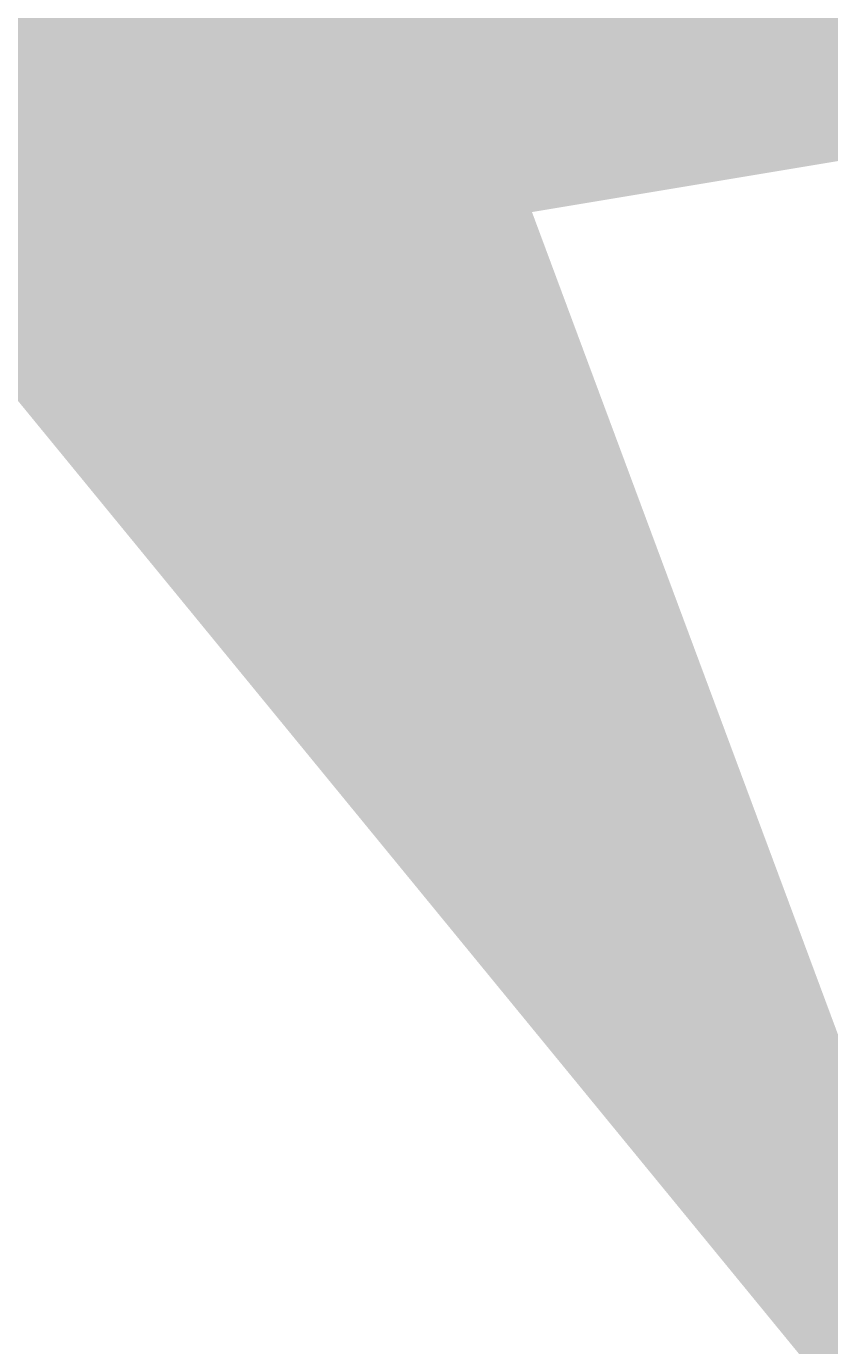
# Model space of a CAD drawing. Units: millimetres. Extents: x -22994 to 29398, y -19990 to 20176.
# Tile 21 of 135: x -44 to 5, y 99 to 180. Entities that reach past the tile are written whole.
import ezdxf

# ---------------------------------------------------------------- set-up
doc = ezdxf.new("R2010")
doc.units = ezdxf.units.MM
doc.header["$MEASUREMENT"] = 0
doc.layers.add('M-DIMS', color=2, linetype='Continuous', lineweight=18)
doc.styles.get("Standard").update_dxf_attribs({"font": 'arial.ttf'})
doc.dimstyles.get("Standard").update_dxf_attribs({"dimtxt": 0.18, "dimasz": 10000, "dimexe": 0.18, "dimexo": 0.0625, "dimgap": 0.09, "dimtad": 0, "dimtih": 1, "dimtoh": 1, "dimdec": 0, "dimzin": 0, "dimdsep": 46, "dimtxsty": 'Standard', "dimcen": 0.09, "dimadec": 0, "dimazin": 0, "dimtfac": 1, "dimtdec": 0, "dimtofl": 0, "dimtmove": 0, "dimatfit": 3, "dimfxl": 1, "dimtolj": 1, "dimtzin": 0, "dimlwd": 30, "dimarcsym": 0})

# ---------------------------------------------------------------- blocks, each defined once
blk = doc.blocks.new('*D2')
at = {"layer": 'Defpoints', "color": 0, "transparency": 16777216}
for p in [(6.677, 10.271), (290.852, 10.271), (290.852, -5.079)]:
    blk.add_point(p, dxfattribs=at)
at = {"layer": 'M-DIMS', "color": 0, "lineweight": -2, "transparency": 16777216}
for p, q in [((6.677, 10.209), (6.677, -5.259)), ((290.852, 10.209), (290.852, -5.259))]:
    blk.add_line(p, q, dxfattribs=at)
at = {"layer": 'M-DIMS', "color": 0, "lineweight": 30, "transparency": 16777216}
for p, q in [((-9993.323, -5.079), (-19993.323, -5.079)), ((10290.852, -5.079), (20290.852, -5.079))]:
    blk.add_line(p, q, dxfattribs=at)
at = {"layer": 'M-DIMS', "color": 0, "transparency": 16777216}
for points in [[(-9993.323, 1661.588), (-9993.323, -1671.745), (6.677, -5.079)], [(10290.852, 1661.588), (10290.852, -1671.745), (290.852, -5.079)]]:
    blk.add_solid(points, dxfattribs=at)
at = {"layer": 'M-DIMS', "color": 0, "transparency": 16777216, "insert": (148.765, -5.079), "char_height": 0.18, "attachment_point": 5}
blk.add_mtext('\\A1;284.2', dxfattribs=at)
blk = doc.blocks.new('*D3')
at = {"layer": 'Defpoints', "color": 0, "transparency": 16777216}
for p in [(110.265, 204.165), (110.265, 176.366), (95.833, 127.967)]:
    blk.add_point(p, dxfattribs=at)
at = {"layer": 'M-DIMS', "color": 0, "lineweight": 30, "transparency": 16777216}
for p, q in [((-9904.167, 204.165), (-19904.167, 204.165)), ((10110.265, 204.165), (20110.265, 204.165))]:
    blk.add_line(p, q, dxfattribs=at)
at = {"layer": 'M-DIMS', "color": 0, "lineweight": -2, "transparency": 16777216}
for p, q in [((95.833, 128.03), (95.833, 204.345)), ((110.265, 176.429), (110.265, 204.345))]:
    blk.add_line(p, q, dxfattribs=at)
at = {"layer": 'M-DIMS', "color": 0, "transparency": 16777216}
for points in [[(-9904.167, 1870.832), (-9904.167, -1462.501), (95.833, 204.165)], [(10110.265, 1870.832), (10110.265, -1462.501), (110.265, 204.165)]]:
    blk.add_solid(points, dxfattribs=at)
at = {"layer": 'M-DIMS', "color": 0, "transparency": 16777216, "insert": (103.049, 204.165), "char_height": 0.18, "attachment_point": 5}
blk.add_mtext('\\A1;14.432', dxfattribs=at)
blk = doc.blocks.new('*D4')
at = {"layer": 'Defpoints', "color": 0, "transparency": 16777216}
for p in [(116.265, 204.165), (110.265, 176.366), (116.265, 176.366)]:
    blk.add_point(p, dxfattribs=at)
at = {"layer": 'M-DIMS', "color": 0, "lineweight": 30, "transparency": 16777216}
for p, q in [((-9889.735, 204.165), (-19889.735, 204.165)), ((10116.265, 204.165), (20116.265, 204.165))]:
    blk.add_line(p, q, dxfattribs=at)
at = {"layer": 'M-DIMS', "color": 0, "lineweight": -2, "transparency": 16777216}
for p, q in [((110.265, 176.429), (110.265, 204.345)), ((116.265, 176.429), (116.265, 204.345))]:
    blk.add_line(p, q, dxfattribs=at)
at = {"layer": 'M-DIMS', "color": 0, "transparency": 16777216}
for points in [[(-9889.735, 1870.832), (-9889.735, -1462.501), (110.265, 204.165)], [(10116.265, 1870.832), (10116.265, -1462.501), (116.265, 204.165)]]:
    blk.add_solid(points, dxfattribs=at)
at = {"layer": 'M-DIMS', "color": 0, "transparency": 16777216, "insert": (113.265, 204.165), "char_height": 0.18, "attachment_point": 5}
blk.add_mtext('\\A1;6', dxfattribs=at)
blk = doc.blocks.new('*D5')
at = {"layer": 'Defpoints', "color": 0, "transparency": 16777216}
for p in [(181.265, 204.165), (116.265, 176.366), (181.265, 176.366)]:
    blk.add_point(p, dxfattribs=at)
at = {"layer": 'M-DIMS', "color": 0, "lineweight": 30, "transparency": 16777216}
for p, q in [((-9883.735, 204.165), (-19883.735, 204.165)), ((10181.265, 204.165), (20181.265, 204.165))]:
    blk.add_line(p, q, dxfattribs=at)
at = {"layer": 'M-DIMS', "color": 0, "lineweight": -2, "transparency": 16777216}
for p, q in [((116.265, 176.429), (116.265, 204.345)), ((181.265, 176.429), (181.265, 204.345))]:
    blk.add_line(p, q, dxfattribs=at)
at = {"layer": 'M-DIMS', "color": 0, "transparency": 16777216}
for points in [[(-9883.735, 1870.832), (-9883.735, -1462.501), (116.265, 204.165)], [(10181.265, 1870.832), (10181.265, -1462.501), (181.265, 204.165)]]:
    blk.add_solid(points, dxfattribs=at)
at = {"layer": 'M-DIMS', "color": 0, "transparency": 16777216, "insert": (148.765, 204.165), "char_height": 0.18, "attachment_point": 5}
blk.add_mtext('\\A1;65', dxfattribs=at)
blk = doc.blocks.new('*D6')
at = {"layer": 'Defpoints', "color": 0, "transparency": 16777216}
for p in [(187.265, 204.165), (181.265, 176.366), (187.265, 176.366)]:
    blk.add_point(p, dxfattribs=at)
at = {"layer": 'M-DIMS', "color": 0, "lineweight": 30, "transparency": 16777216}
for p, q in [((-9818.735, 204.165), (-19818.735, 204.165)), ((10187.265, 204.165), (20187.265, 204.165))]:
    blk.add_line(p, q, dxfattribs=at)
at = {"layer": 'M-DIMS', "color": 0, "lineweight": -2, "transparency": 16777216}
for p, q in [((181.265, 176.429), (181.265, 204.345)), ((187.265, 176.429), (187.265, 204.345))]:
    blk.add_line(p, q, dxfattribs=at)
at = {"layer": 'M-DIMS', "color": 0, "transparency": 16777216}
for points in [[(-9818.735, 1870.832), (-9818.735, -1462.501), (181.265, 204.165)], [(10187.265, 1870.832), (10187.265, -1462.501), (187.265, 204.165)]]:
    blk.add_solid(points, dxfattribs=at)
at = {"layer": 'M-DIMS', "color": 0, "transparency": 16777216, "insert": (184.265, 204.165), "char_height": 0.18, "attachment_point": 5}
blk.add_mtext('\\A1;6', dxfattribs=at)
blk = doc.blocks.new('*D7')
at = {"layer": 'Defpoints', "color": 0, "transparency": 16777216}
for p in [(201.697, 204.165), (187.265, 176.366), (201.697, 127.967)]:
    blk.add_point(p, dxfattribs=at)
at = {"layer": 'M-DIMS', "color": 0, "lineweight": 30, "transparency": 16777216}
for p, q in [((-9812.735, 204.165), (-19812.735, 204.165)), ((10201.697, 204.165), (20201.697, 204.165))]:
    blk.add_line(p, q, dxfattribs=at)
at = {"layer": 'M-DIMS', "color": 0, "lineweight": -2, "transparency": 16777216}
for p, q in [((187.265, 176.429), (187.265, 204.345)), ((201.697, 128.03), (201.697, 204.345))]:
    blk.add_line(p, q, dxfattribs=at)
at = {"layer": 'M-DIMS', "color": 0, "transparency": 16777216}
for points in [[(-9812.735, 1870.832), (-9812.735, -1462.501), (187.265, 204.165)], [(10201.697, 1870.832), (10201.697, -1462.501), (201.697, 204.165)]]:
    blk.add_solid(points, dxfattribs=at)
at = {"layer": 'M-DIMS', "color": 0, "transparency": 16777216, "insert": (194.481, 204.165), "char_height": 0.18, "attachment_point": 5}
blk.add_mtext('\\A1;14.432', dxfattribs=at)
blk = doc.blocks.new('*D8')
at = {"layer": 'Defpoints', "color": 0, "transparency": 16777216}
for p in [(227.648, 204.165), (227.648, 146.73), (201.697, 127.967)]:
    blk.add_point(p, dxfattribs=at)
at = {"layer": 'M-DIMS', "color": 0, "lineweight": 30, "transparency": 16777216}
for p, q in [((-9798.303, 204.165), (-19798.303, 204.165)), ((10227.648, 204.165), (20227.648, 204.165))]:
    blk.add_line(p, q, dxfattribs=at)
at = {"layer": 'M-DIMS', "color": 0, "lineweight": -2, "transparency": 16777216}
for p, q in [((201.697, 128.03), (201.697, 204.345)), ((227.648, 146.792), (227.648, 204.345))]:
    blk.add_line(p, q, dxfattribs=at)
at = {"layer": 'M-DIMS', "color": 0, "transparency": 16777216}
for points in [[(-9798.303, 1870.832), (-9798.303, -1462.501), (201.697, 204.165)], [(10227.648, 1870.832), (10227.648, -1462.501), (227.648, 204.165)]]:
    blk.add_solid(points, dxfattribs=at)
at = {"layer": 'M-DIMS', "color": 0, "transparency": 16777216, "insert": (214.673, 204.165), "char_height": 0.18, "attachment_point": 5}
blk.add_mtext('\\A1;25.95', dxfattribs=at)
blk = doc.blocks.new('*D9')
at = {"layer": 'Defpoints', "color": 0, "transparency": 16777216}
for p in [(187.265, 176.366), (306.202, 176.366), (290.852, 10.271)]:
    blk.add_point(p, dxfattribs=at)
at = {"layer": 'M-DIMS', "color": 0, "lineweight": 30, "transparency": 16777216}
for p, q in [((306.202, 10176.366), (306.202, 20176.366)), ((306.202, -9989.729), (306.202, -19989.729))]:
    blk.add_line(p, q, dxfattribs=at)
at = {"layer": 'M-DIMS', "color": 0, "lineweight": -2, "transparency": 16777216}
for p, q in [((187.327, 176.366), (306.382, 176.366)), ((290.915, 10.271), (306.382, 10.271))]:
    blk.add_line(p, q, dxfattribs=at)
at = {"layer": 'M-DIMS', "color": 0, "transparency": 16777216}
for points in [[(-1360.465, 10176.366), (1972.869, 10176.366), (306.202, 176.366)], [(-1360.465, -9989.729), (1972.869, -9989.729), (306.202, 10.271)]]:
    blk.add_solid(points, dxfattribs=at)
at = {"layer": 'M-DIMS', "color": 0, "transparency": 16777216, "insert": (306.202, 93.319), "char_height": 0.18, "attachment_point": 5}
blk.add_mtext('\\A1;166.1', dxfattribs=at)
blk = doc.blocks.new('*D10')
at = {"layer": 'Defpoints', "color": 0, "transparency": 16777216}
for p in [(125.65, 136.071), (133.346, 136.071), (133.346, -5.079)]:
    blk.add_point(p, dxfattribs=at)
at = {"layer": 'M-DIMS', "color": 0, "lineweight": -2, "transparency": 16777216}
for p, q in [((125.65, 136.009), (125.65, -5.259)), ((133.346, 136.009), (133.346, -5.259))]:
    blk.add_line(p, q, dxfattribs=at)
at = {"layer": 'M-DIMS', "color": 0, "lineweight": 30, "transparency": 16777216}
for p, q in [((-9874.35, -5.079), (-19874.35, -5.079)), ((10133.346, -5.079), (20133.346, -5.079))]:
    blk.add_line(p, q, dxfattribs=at)
at = {"layer": 'M-DIMS', "color": 0, "transparency": 16777216}
for points in [[(-9874.35, 1661.588), (-9874.35, -1671.745), (125.65, -5.079)], [(10133.346, 1661.588), (10133.346, -1671.745), (133.346, -5.079)]]:
    blk.add_solid(points, dxfattribs=at)
at = {"layer": 'M-DIMS', "color": 0, "transparency": 16777216, "insert": (129.498, -5.079), "char_height": 0.18, "attachment_point": 5}
blk.add_mtext('\\A1;7.696', dxfattribs=at)
blk = doc.blocks.new('*D11')
at = {"layer": 'Defpoints', "color": 0, "transparency": 16777216}
for p in [(133.346, 136.071), (135.65, 136.071), (135.65, -5.079)]:
    blk.add_point(p, dxfattribs=at)
at = {"layer": 'M-DIMS', "color": 0, "lineweight": -2, "transparency": 16777216}
for p, q in [((133.346, 136.009), (133.346, -5.259)), ((135.65, 136.009), (135.65, -5.259))]:
    blk.add_line(p, q, dxfattribs=at)
at = {"layer": 'M-DIMS', "color": 0, "lineweight": 30, "transparency": 16777216}
for p, q in [((-9866.654, -5.079), (-19866.654, -5.079)), ((10135.65, -5.079), (20135.65, -5.079))]:
    blk.add_line(p, q, dxfattribs=at)
at = {"layer": 'M-DIMS', "color": 0, "transparency": 16777216}
for points in [[(-9866.654, 1661.588), (-9866.654, -1671.745), (133.346, -5.079)], [(10135.65, 1661.588), (10135.65, -1671.745), (135.65, -5.079)]]:
    blk.add_solid(points, dxfattribs=at)
at = {"layer": 'M-DIMS', "color": 0, "transparency": 16777216, "insert": (134.498, -5.079), "char_height": 0.18, "attachment_point": 5}
blk.add_mtext('\\A1;2.304', dxfattribs=at)
blk = doc.blocks.new('*D12')
at = {"layer": 'Defpoints', "color": 0, "transparency": 16777216}
for p in [(135.65, 136.071), (145.65, 136.071), (145.65, -5.079)]:
    blk.add_point(p, dxfattribs=at)
at = {"layer": 'M-DIMS', "color": 0, "lineweight": -2, "transparency": 16777216}
for p, q in [((135.65, 136.009), (135.65, -5.259)), ((145.65, 136.009), (145.65, -5.259))]:
    blk.add_line(p, q, dxfattribs=at)
at = {"layer": 'M-DIMS', "color": 0, "lineweight": 30, "transparency": 16777216}
for p, q in [((-9864.35, -5.079), (-19864.35, -5.079)), ((10145.65, -5.079), (20145.65, -5.079))]:
    blk.add_line(p, q, dxfattribs=at)
at = {"layer": 'M-DIMS', "color": 0, "transparency": 16777216}
for points in [[(-9864.35, 1661.588), (-9864.35, -1671.745), (135.65, -5.079)], [(10145.65, 1661.588), (10145.65, -1671.745), (145.65, -5.079)]]:
    blk.add_solid(points, dxfattribs=at)
at = {"layer": 'M-DIMS', "color": 0, "transparency": 16777216, "insert": (140.65, -5.079), "char_height": 0.18, "attachment_point": 5}
blk.add_mtext('\\A1;10', dxfattribs=at)
blk = doc.blocks.new('*D13')
at = {"layer": 'Defpoints', "color": 0, "transparency": 16777216}
for p in [(145.65, 136.071), (155.65, 136.071), (155.65, -5.079)]:
    blk.add_point(p, dxfattribs=at)
at = {"layer": 'M-DIMS', "color": 0, "lineweight": -2, "transparency": 16777216}
for p, q in [((145.65, 136.009), (145.65, -5.259)), ((155.65, 136.009), (155.65, -5.259))]:
    blk.add_line(p, q, dxfattribs=at)
at = {"layer": 'M-DIMS', "color": 0, "lineweight": 30, "transparency": 16777216}
for p, q in [((-9854.35, -5.079), (-19854.35, -5.079)), ((10155.65, -5.079), (20155.65, -5.079))]:
    blk.add_line(p, q, dxfattribs=at)
at = {"layer": 'M-DIMS', "color": 0, "transparency": 16777216}
for points in [[(-9854.35, 1661.588), (-9854.35, -1671.745), (145.65, -5.079)], [(10155.65, 1661.588), (10155.65, -1671.745), (155.65, -5.079)]]:
    blk.add_solid(points, dxfattribs=at)
at = {"layer": 'M-DIMS', "color": 0, "transparency": 16777216, "insert": (150.65, -5.079), "char_height": 0.18, "attachment_point": 5}
blk.add_mtext('\\A1;10', dxfattribs=at)
blk = doc.blocks.new('*D14')
at = {"layer": 'Defpoints', "color": 0, "transparency": 16777216}
for p in [(155.65, 136.071), (165.65, 136.071), (165.65, -5.079)]:
    blk.add_point(p, dxfattribs=at)
at = {"layer": 'M-DIMS', "color": 0, "lineweight": -2, "transparency": 16777216}
for p, q in [((155.65, 136.009), (155.65, -5.259)), ((165.65, 136.009), (165.65, -5.259))]:
    blk.add_line(p, q, dxfattribs=at)
at = {"layer": 'M-DIMS', "color": 0, "lineweight": 30, "transparency": 16777216}
for p, q in [((-9844.35, -5.079), (-19844.35, -5.079)), ((10165.65, -5.079), (20165.65, -5.079))]:
    blk.add_line(p, q, dxfattribs=at)
at = {"layer": 'M-DIMS', "color": 0, "transparency": 16777216}
for points in [[(-9844.35, 1661.588), (-9844.35, -1671.745), (155.65, -5.079)], [(10165.65, 1661.588), (10165.65, -1671.745), (165.65, -5.079)]]:
    blk.add_solid(points, dxfattribs=at)
at = {"layer": 'M-DIMS', "color": 0, "transparency": 16777216, "insert": (160.65, -5.079), "char_height": 0.18, "attachment_point": 5}
blk.add_mtext('\\A1;10', dxfattribs=at)
blk = doc.blocks.new('*D15')
at = {"layer": 'Defpoints', "color": 0, "transparency": 16777216}
for p in [(173.346, 154.788), (173.346, 136.071), (306.202, 136.071)]:
    blk.add_point(p, dxfattribs=at)
at = {"layer": 'M-DIMS', "color": 0, "lineweight": 30, "transparency": 16777216}
for p, q in [((306.202, 10154.788), (306.202, 20154.788)), ((306.202, -9863.929), (306.202, -19863.929))]:
    blk.add_line(p, q, dxfattribs=at)
at = {"layer": 'M-DIMS', "color": 0, "lineweight": -2, "transparency": 16777216}
for p, q in [((173.408, 154.788), (306.382, 154.788)), ((173.408, 136.071), (306.382, 136.071))]:
    blk.add_line(p, q, dxfattribs=at)
at = {"layer": 'M-DIMS', "color": 0, "transparency": 16777216}
for points in [[(-1360.465, 10154.788), (1972.869, 10154.788), (306.202, 154.788)], [(-1360.465, -9863.929), (1972.869, -9863.929), (306.202, 136.071)]]:
    blk.add_solid(points, dxfattribs=at)
at = {"layer": 'M-DIMS', "color": 0, "transparency": 16777216, "insert": (306.202, 145.43), "char_height": 0.18, "attachment_point": 5}
blk.add_mtext('\\A1;18.717', dxfattribs=at)
blk = doc.blocks.new('*D16')
at = {"layer": 'Defpoints', "color": 0, "transparency": 16777216}
for p in [(120.17, 204.165), (110.466, 48.035), (120.17, 48.035)]:
    blk.add_point(p, dxfattribs=at)
at = {"layer": 'M-DIMS', "color": 0, "lineweight": 30, "transparency": 16777216}
for p, q in [((-9889.534, 204.165), (-19889.534, 204.165)), ((10120.17, 204.165), (20120.17, 204.165))]:
    blk.add_line(p, q, dxfattribs=at)
at = {"layer": 'M-DIMS', "color": 0, "lineweight": -2, "transparency": 16777216}
for p, q in [((110.466, 48.097), (110.466, 204.345)), ((120.17, 48.097), (120.17, 204.345))]:
    blk.add_line(p, q, dxfattribs=at)
at = {"layer": 'M-DIMS', "color": 0, "transparency": 16777216}
for points in [[(-9889.534, 1870.832), (-9889.534, -1462.501), (110.466, 204.165)], [(10120.17, 1870.832), (10120.17, -1462.501), (120.17, 204.165)]]:
    blk.add_solid(points, dxfattribs=at)
at = {"layer": 'M-DIMS', "color": 0, "transparency": 16777216, "insert": (115.318, 204.165), "char_height": 0.18, "attachment_point": 5}
blk.add_mtext('\\A1;9.704', dxfattribs=at)
blk = doc.blocks.new('*D17')
at = {"layer": 'Defpoints', "color": 0, "transparency": 16777216}
for p in [(126.17, 204.165), (120.17, 48.035), (126.17, 48.035)]:
    blk.add_point(p, dxfattribs=at)
at = {"layer": 'M-DIMS', "color": 0, "lineweight": 30, "transparency": 16777216}
for p, q in [((-9879.83, 204.165), (-19879.83, 204.165)), ((10126.17, 204.165), (20126.17, 204.165))]:
    blk.add_line(p, q, dxfattribs=at)
at = {"layer": 'M-DIMS', "color": 0, "lineweight": -2, "transparency": 16777216}
for p, q in [((120.17, 48.097), (120.17, 204.345)), ((126.17, 48.097), (126.17, 204.345))]:
    blk.add_line(p, q, dxfattribs=at)
at = {"layer": 'M-DIMS', "color": 0, "transparency": 16777216}
for points in [[(-9879.83, 1870.832), (-9879.83, -1462.501), (120.17, 204.165)], [(10126.17, 1870.832), (10126.17, -1462.501), (126.17, 204.165)]]:
    blk.add_solid(points, dxfattribs=at)
at = {"layer": 'M-DIMS', "color": 0, "transparency": 16777216, "insert": (123.17, 204.165), "char_height": 0.18, "attachment_point": 5}
blk.add_mtext('\\A1;6', dxfattribs=at)
blk = doc.blocks.new('*D18')
at = {"layer": 'Defpoints', "color": 0, "transparency": 16777216}
for p in [(132.17, 204.165), (126.17, 48.035), (132.17, 48.035)]:
    blk.add_point(p, dxfattribs=at)
at = {"layer": 'M-DIMS', "color": 0, "lineweight": 30, "transparency": 16777216}
for p, q in [((-9873.83, 204.165), (-19873.83, 204.165)), ((10132.17, 204.165), (20132.17, 204.165))]:
    blk.add_line(p, q, dxfattribs=at)
at = {"layer": 'M-DIMS', "color": 0, "lineweight": -2, "transparency": 16777216}
for p, q in [((126.17, 48.097), (126.17, 204.345)), ((132.17, 48.097), (132.17, 204.345))]:
    blk.add_line(p, q, dxfattribs=at)
at = {"layer": 'M-DIMS', "color": 0, "transparency": 16777216}
for points in [[(-9873.83, 1870.832), (-9873.83, -1462.501), (126.17, 204.165)], [(10132.17, 1870.832), (10132.17, -1462.501), (132.17, 204.165)]]:
    blk.add_solid(points, dxfattribs=at)
at = {"layer": 'M-DIMS', "color": 0, "transparency": 16777216, "insert": (129.17, 204.165), "char_height": 0.18, "attachment_point": 5}
blk.add_mtext('\\A1;6', dxfattribs=at)
blk = doc.blocks.new('*D19')
at = {"layer": 'Defpoints', "color": 0, "transparency": 16777216}
for p in [(138.17, 204.165), (132.17, 48.035), (138.17, 48.035)]:
    blk.add_point(p, dxfattribs=at)
at = {"layer": 'M-DIMS', "color": 0, "lineweight": 30, "transparency": 16777216}
for p, q in [((-9867.83, 204.165), (-19867.83, 204.165)), ((10138.17, 204.165), (20138.17, 204.165))]:
    blk.add_line(p, q, dxfattribs=at)
at = {"layer": 'M-DIMS', "color": 0, "lineweight": -2, "transparency": 16777216}
for p, q in [((132.17, 48.097), (132.17, 204.345)), ((138.17, 48.097), (138.17, 204.345))]:
    blk.add_line(p, q, dxfattribs=at)
at = {"layer": 'M-DIMS', "color": 0, "transparency": 16777216}
for points in [[(-9867.83, 1870.832), (-9867.83, -1462.501), (132.17, 204.165)], [(10138.17, 1870.832), (10138.17, -1462.501), (138.17, 204.165)]]:
    blk.add_solid(points, dxfattribs=at)
at = {"layer": 'M-DIMS', "color": 0, "transparency": 16777216, "insert": (135.17, 204.165), "char_height": 0.18, "attachment_point": 5}
blk.add_mtext('\\A1;6', dxfattribs=at)
blk = doc.blocks.new('*D20')
at = {"layer": 'Defpoints', "color": 0, "transparency": 16777216}
for p in [(144.17, 204.165), (138.17, 48.035), (144.17, 48.035)]:
    blk.add_point(p, dxfattribs=at)
at = {"layer": 'M-DIMS', "color": 0, "lineweight": 30, "transparency": 16777216}
for p, q in [((-9861.83, 204.165), (-19861.83, 204.165)), ((10144.17, 204.165), (20144.17, 204.165))]:
    blk.add_line(p, q, dxfattribs=at)
at = {"layer": 'M-DIMS', "color": 0, "lineweight": -2, "transparency": 16777216}
for p, q in [((138.17, 48.097), (138.17, 204.345)), ((144.17, 48.097), (144.17, 204.345))]:
    blk.add_line(p, q, dxfattribs=at)
at = {"layer": 'M-DIMS', "color": 0, "transparency": 16777216}
for points in [[(-9861.83, 1870.832), (-9861.83, -1462.501), (138.17, 204.165)], [(10144.17, 1870.832), (10144.17, -1462.501), (144.17, 204.165)]]:
    blk.add_solid(points, dxfattribs=at)
at = {"layer": 'M-DIMS', "color": 0, "transparency": 16777216, "insert": (141.17, 204.165), "char_height": 0.18, "attachment_point": 5}
blk.add_mtext('\\A1;6', dxfattribs=at)
blk = doc.blocks.new('*D21')
at = {"layer": 'Defpoints', "color": 0, "transparency": 16777216}
for p in [(149.116, 204.165), (144.17, 48.035), (149.116, 48.035)]:
    blk.add_point(p, dxfattribs=at)
at = {"layer": 'M-DIMS', "color": 0, "lineweight": 30, "transparency": 16777216}
for p, q in [((-9855.83, 204.165), (-19855.83, 204.165)), ((10149.116, 204.165), (20149.116, 204.165))]:
    blk.add_line(p, q, dxfattribs=at)
at = {"layer": 'M-DIMS', "color": 0, "lineweight": -2, "transparency": 16777216}
for p, q in [((144.17, 48.097), (144.17, 204.345)), ((149.116, 48.097), (149.116, 204.345))]:
    blk.add_line(p, q, dxfattribs=at)
at = {"layer": 'M-DIMS', "color": 0, "transparency": 16777216}
for points in [[(-9855.83, 1870.832), (-9855.83, -1462.501), (144.17, 204.165)], [(10149.116, 1870.832), (10149.116, -1462.501), (149.116, 204.165)]]:
    blk.add_solid(points, dxfattribs=at)
at = {"layer": 'M-DIMS', "color": 0, "transparency": 16777216, "insert": (146.643, 204.165), "char_height": 0.18, "attachment_point": 5}
blk.add_mtext('\\A1;4.945', dxfattribs=at)
blk = doc.blocks.new('*D22')
at = {"layer": 'Defpoints', "color": 0, "transparency": 16777216}
for p in [(149.116, 30.99), (155.116, 30.99), (155.116, -5.079)]:
    blk.add_point(p, dxfattribs=at)
at = {"layer": 'M-DIMS', "color": 0, "lineweight": -2, "transparency": 16777216}
for p, q in [((149.116, 30.927), (149.116, -5.259)), ((155.116, 30.927), (155.116, -5.259))]:
    blk.add_line(p, q, dxfattribs=at)
at = {"layer": 'M-DIMS', "color": 0, "lineweight": 30, "transparency": 16777216}
for p, q in [((-9850.884, -5.079), (-19850.884, -5.079)), ((10155.116, -5.079), (20155.116, -5.079))]:
    blk.add_line(p, q, dxfattribs=at)
at = {"layer": 'M-DIMS', "color": 0, "transparency": 16777216}
for points in [[(-9850.884, 1661.588), (-9850.884, -1671.745), (149.116, -5.079)], [(10155.116, 1661.588), (10155.116, -1671.745), (155.116, -5.079)]]:
    blk.add_solid(points, dxfattribs=at)
at = {"layer": 'M-DIMS', "color": 0, "transparency": 16777216, "insert": (152.116, -5.079), "char_height": 0.18, "attachment_point": 5}
blk.add_mtext('\\A1;6', dxfattribs=at)
blk = doc.blocks.new('*D23')
at = {"layer": 'Defpoints', "color": 0, "transparency": 16777216}
for p in [(155.116, 30.99), (161.116, 30.99), (161.116, -5.079)]:
    blk.add_point(p, dxfattribs=at)
at = {"layer": 'M-DIMS', "color": 0, "lineweight": -2, "transparency": 16777216}
for p, q in [((155.116, 30.927), (155.116, -5.259)), ((161.116, 30.927), (161.116, -5.259))]:
    blk.add_line(p, q, dxfattribs=at)
at = {"layer": 'M-DIMS', "color": 0, "lineweight": 30, "transparency": 16777216}
for p, q in [((-9844.884, -5.079), (-19844.884, -5.079)), ((10161.116, -5.079), (20161.116, -5.079))]:
    blk.add_line(p, q, dxfattribs=at)
at = {"layer": 'M-DIMS', "color": 0, "transparency": 16777216}
for points in [[(-9844.884, 1661.588), (-9844.884, -1671.745), (155.116, -5.079)], [(10161.116, 1661.588), (10161.116, -1671.745), (161.116, -5.079)]]:
    blk.add_solid(points, dxfattribs=at)
at = {"layer": 'M-DIMS', "color": 0, "transparency": 16777216, "insert": (158.116, -5.079), "char_height": 0.18, "attachment_point": 5}
blk.add_mtext('\\A1;6', dxfattribs=at)
blk = doc.blocks.new('*D24')
at = {"layer": 'Defpoints', "color": 0, "transparency": 16777216}
for p in [(161.116, 30.99), (166.439, 30.99), (166.439, -5.079)]:
    blk.add_point(p, dxfattribs=at)
at = {"layer": 'M-DIMS', "color": 0, "lineweight": -2, "transparency": 16777216}
for p, q in [((161.116, 30.927), (161.116, -5.259)), ((166.439, 30.927), (166.439, -5.259))]:
    blk.add_line(p, q, dxfattribs=at)
at = {"layer": 'M-DIMS', "color": 0, "lineweight": 30, "transparency": 16777216}
for p, q in [((-9838.884, -5.079), (-19838.884, -5.079)), ((10166.439, -5.079), (20166.439, -5.079))]:
    blk.add_line(p, q, dxfattribs=at)
at = {"layer": 'M-DIMS', "color": 0, "transparency": 16777216}
for points in [[(-9838.884, 1661.588), (-9838.884, -1671.745), (161.116, -5.079)], [(10166.439, 1661.588), (10166.439, -1671.745), (166.439, -5.079)]]:
    blk.add_solid(points, dxfattribs=at)
at = {"layer": 'M-DIMS', "color": 0, "transparency": 16777216, "insert": (163.777, -5.079), "char_height": 0.18, "attachment_point": 5}
blk.add_mtext('\\A1;5.323', dxfattribs=at)
blk = doc.blocks.new('*D25')
at = {"layer": 'Defpoints', "color": 0, "transparency": 16777216}
for p in [(166.439, 30.99), (172.439, 30.99), (172.439, -5.079)]:
    blk.add_point(p, dxfattribs=at)
at = {"layer": 'M-DIMS', "color": 0, "lineweight": -2, "transparency": 16777216}
for p, q in [((166.439, 30.927), (166.439, -5.259)), ((172.439, 30.927), (172.439, -5.259))]:
    blk.add_line(p, q, dxfattribs=at)
at = {"layer": 'M-DIMS', "color": 0, "lineweight": 30, "transparency": 16777216}
for p, q in [((-9833.561, -5.079), (-19833.561, -5.079)), ((10172.439, -5.079), (20172.439, -5.079))]:
    blk.add_line(p, q, dxfattribs=at)
at = {"layer": 'M-DIMS', "color": 0, "transparency": 16777216}
for points in [[(-9833.561, 1661.588), (-9833.561, -1671.745), (166.439, -5.079)], [(10172.439, 1661.588), (10172.439, -1671.745), (172.439, -5.079)]]:
    blk.add_solid(points, dxfattribs=at)
at = {"layer": 'M-DIMS', "color": 0, "transparency": 16777216, "insert": (169.439, -5.079), "char_height": 0.18, "attachment_point": 5}
blk.add_mtext('\\A1;6', dxfattribs=at)
blk = doc.blocks.new('*D26')
at = {"layer": 'Defpoints', "color": 0, "transparency": 16777216}
for p in [(172.439, 30.99), (178.439, 30.99), (178.439, -5.079)]:
    blk.add_point(p, dxfattribs=at)
at = {"layer": 'M-DIMS', "color": 0, "lineweight": -2, "transparency": 16777216}
for p, q in [((172.439, 30.927), (172.439, -5.259)), ((178.439, 30.927), (178.439, -5.259))]:
    blk.add_line(p, q, dxfattribs=at)
at = {"layer": 'M-DIMS', "color": 0, "lineweight": 30, "transparency": 16777216}
for p, q in [((-9827.561, -5.079), (-19827.561, -5.079)), ((10178.439, -5.079), (20178.439, -5.079))]:
    blk.add_line(p, q, dxfattribs=at)
at = {"layer": 'M-DIMS', "color": 0, "transparency": 16777216}
for points in [[(-9827.561, 1661.588), (-9827.561, -1671.745), (172.439, -5.079)], [(10178.439, 1661.588), (10178.439, -1671.745), (178.439, -5.079)]]:
    blk.add_solid(points, dxfattribs=at)
at = {"layer": 'M-DIMS', "color": 0, "transparency": 16777216, "insert": (175.439, -5.079), "char_height": 0.18, "attachment_point": 5}
blk.add_mtext('\\A1;6', dxfattribs=at)
blk = doc.blocks.new('*D27')
at = {"layer": 'Defpoints', "color": 0, "transparency": 16777216}
for p in [(178.439, 30.99), (188.117, 30.99), (188.117, -5.079)]:
    blk.add_point(p, dxfattribs=at)
at = {"layer": 'M-DIMS', "color": 0, "lineweight": -2, "transparency": 16777216}
for p, q in [((178.439, 30.927), (178.439, -5.259)), ((188.117, 30.927), (188.117, -5.259))]:
    blk.add_line(p, q, dxfattribs=at)
at = {"layer": 'M-DIMS', "color": 0, "lineweight": 30, "transparency": 16777216}
for p, q in [((-9821.561, -5.079), (-19821.561, -5.079)), ((10188.117, -5.079), (20188.117, -5.079))]:
    blk.add_line(p, q, dxfattribs=at)
at = {"layer": 'M-DIMS', "color": 0, "transparency": 16777216}
for points in [[(-9821.561, 1661.588), (-9821.561, -1671.745), (178.439, -5.079)], [(10188.117, 1661.588), (10188.117, -1671.745), (188.117, -5.079)]]:
    blk.add_solid(points, dxfattribs=at)
at = {"layer": 'M-DIMS', "color": 0, "transparency": 16777216, "insert": (183.278, -5.079), "char_height": 0.18, "attachment_point": 5}
blk.add_mtext('\\A1;9.679', dxfattribs=at)
blk = doc.blocks.new('*D28')
at = {"layer": 'Defpoints', "color": 0, "transparency": 16777216}
for p in [(188.117, 48.035), (306.202, 48.035), (188.117, 30.99)]:
    blk.add_point(p, dxfattribs=at)
at = {"layer": 'M-DIMS', "color": 0, "lineweight": 30, "transparency": 16777216}
for p, q in [((306.202, 10048.035), (306.202, 20048.035)), ((306.202, -9969.01), (306.202, -19969.01))]:
    blk.add_line(p, q, dxfattribs=at)
at = {"layer": 'M-DIMS', "color": 0, "lineweight": -2, "transparency": 16777216}
for p, q in [((188.18, 48.035), (306.382, 48.035)), ((188.18, 30.99), (306.382, 30.99))]:
    blk.add_line(p, q, dxfattribs=at)
at = {"layer": 'M-DIMS', "color": 0, "transparency": 16777216}
for points in [[(-1360.465, 10048.035), (1972.869, 10048.035), (306.202, 48.035)], [(-1360.465, -9969.01), (1972.869, -9969.01), (306.202, 30.99)]]:
    blk.add_solid(points, dxfattribs=at)
at = {"layer": 'M-DIMS', "color": 0, "transparency": 16777216, "insert": (306.202, 39.512), "char_height": 0.18, "attachment_point": 5}
blk.add_mtext('\\A1;17.045', dxfattribs=at)
blk = doc.blocks.new('*D32')
at = {"layer": 'Defpoints', "color": 0, "transparency": 16777216}
for p in [(57.164, 118.614), (52.413, 113.093)]:
    blk.add_point(p, dxfattribs=at)
at = {"layer": 'M-DIMS', "color": 0, "lineweight": -2, "transparency": 16777216}
for p, q in [((57.074, 118.614), (57.254, 118.614)), ((57.164, 118.524), (57.164, 118.704))]:
    blk.add_line(p, q, dxfattribs=at)
at = {"layer": 'M-DIMS', "color": 0, "lineweight": 30, "transparency": 16777216}
for p, q in [((-12992.534, -15047.031), (-6470.06, -7466.969)), ((-22992.534, -15047.031), (-12992.534, -15047.031))]:
    blk.add_line(p, q, dxfattribs=at)
at = {"layer": 'M-DIMS', "color": 0, "transparency": 16777216}
blk.add_solid([(-7733.404, -6379.89), (-5206.717, -8554.048), (52.413, 113.093)], dxfattribs=at)
at = {"layer": 'M-DIMS', "color": 0, "transparency": 16777216, "insert": (-22993.208, -15047.031), "char_height": 0.18, "attachment_point": 5}
blk.add_mtext('\\A1;2X R7.284', dxfattribs=at)
blk = doc.blocks.new('*D35')
at = {"layer": 'Defpoints', "color": 0, "transparency": 16777216}
for p in [(21.093, 77.393), (21.84, 76.092)]:
    blk.add_point(p, dxfattribs=at)
at = {"layer": 'M-DIMS', "color": 0, "lineweight": 30, "transparency": 16777216}
for p, q in [((-19938.013, 17421.447), (-9938.013, 17421.447)), ((-9938.013, 17421.447), (-4958.46, 8749.42))]:
    blk.add_line(p, q, dxfattribs=at)
at = {"layer": 'M-DIMS', "color": 0, "lineweight": -2, "transparency": 16777216}
for p, q in [((21.75, 76.092), (21.93, 76.092)), ((21.84, 76.002), (21.84, 76.182))]:
    blk.add_line(p, q, dxfattribs=at)
at = {"layer": 'M-DIMS', "color": 0, "transparency": 16777216}
blk.add_solid([(-3513.122, 9579.345), (-6403.798, 7919.494), (21.093, 77.393)], dxfattribs=at)
at = {"layer": 'M-DIMS', "color": 0, "transparency": 16777216, "insert": (-19938.354, 17421.447), "char_height": 0.18, "attachment_point": 5}
blk.add_mtext('\\A1;R1.5', dxfattribs=at)
blk = doc.blocks.new('*D36')
at = {"layer": 'Defpoints', "color": 0, "transparency": 16777216}
for p in [(46.39, 31.303), (46.387, 26.593)]:
    blk.add_point(p, dxfattribs=at)
at = {"layer": 'M-DIMS', "color": 0, "lineweight": 30, "transparency": 16777216}
for p, q in [((57.15, 20031.301), (51.77, 10031.302)), ((10057.15, 20031.301), (57.15, 20031.301))]:
    blk.add_line(p, q, dxfattribs=at)
at = {"layer": 'M-DIMS', "color": 0, "lineweight": -2, "transparency": 16777216}
for p, q in [((46.299, 28.948), (46.479, 28.948)), ((46.389, 28.858), (46.389, 29.038))]:
    blk.add_line(p, q, dxfattribs=at)
at = {"layer": 'M-DIMS', "color": 0, "transparency": 16777216}
blk.add_solid([(-1614.896, 10032.199), (1718.436, 10030.405), (46.39, 31.303)], dxfattribs=at)
at = {"layer": 'M-DIMS', "color": 0, "transparency": 16777216, "insert": (10057.554, 20031.301), "char_height": 0.18, "attachment_point": 5}
blk.add_mtext('\\A1;∅4.71', dxfattribs=at)

msp = doc.modelspace()

# ---------------------------------------------------------------- dimensions: what is measured, and where the dimension line sits
at = {"layer": 'M-DIMS'}
for base, p1, p2, override, picture, middle in [((306.202, 176.3662), (290.852, 10.2713), (187.2647, 176.3662), {"dimdec": 1, "dimlfac": 1, "dimrnd": 0, "dimzin": 0, "dimdsep": 46, "dimlunit": 2}, '*D9', (306.202, 93.3187)), ((306.202, 136.0713), (173.3459, 154.788), (173.3459, 136.0713), {"dimdec": 3, "dimlfac": 1, "dimrnd": 0, "dimzin": 0, "dimdsep": 46, "dimlunit": 2}, '*D15', (306.202, 145.4297)), ((306.202, 48.0349), (188.1175, 30.9895), (188.1175, 48.0349), {"dimdec": 3, "dimlfac": 1, "dimrnd": 0, "dimzin": 0, "dimdsep": 46, "dimlunit": 2}, '*D28', (306.202, 39.5122))]:
    dim = msp.add_linear_dim(base=base, p1=p1, p2=p2, angle=90, dimstyle='Standard', override=override, dxfattribs=at)
    dim.commit()
    dim.dimension.update_dxf_attribs({"geometry": picture, "text_midpoint": middle})
dim = msp.add_diameter_dim_2p(p1=(46.3875, 26.5934), p2=(46.39, 31.3035), dimstyle='Standard', override={"dimdec": 2, "dimlfac": 1, "dimrnd": 0, "dimzin": 0, "dimdsep": 46, "dimlunit": 2}, dxfattribs=at)
dim.commit()
dim.dimension.update_dxf_attribs({"geometry": '*D36', "text_midpoint": (10057.5542, 20031.3006), "dimtype": 163})
dim = msp.add_radius_dim(center=(21.8402, 76.0922), mpoint=(21.0933, 77.393), dimstyle='Standard', override={"dimdec": 1, "dimlfac": 1, "dimrnd": 0, "dimzin": 0, "dimdsep": 46, "dimlunit": 2}, dxfattribs=at)
dim.commit()
dim.dimension.update_dxf_attribs({"geometry": '*D35', "text_midpoint": (-19938.3541, 17421.4466)})
for base, p1, p2, override, picture, middle in [((110.2647, 204.1654), (95.8327, 127.967), (110.2647, 176.3662), {"dimdec": 3, "dimlfac": 1, "dimrnd": 0, "dimzin": 0, "dimdsep": 46, "dimlunit": 2}, '*D3', (103.0487, 204.1654)), ((116.2647, 204.1654), (110.2647, 176.3662), (116.2647, 176.3662), {"dimdec": 0, "dimlfac": 1, "dimrnd": 0, "dimzin": 0, "dimdsep": 46, "dimlunit": 2}, '*D4', (113.2647, 204.1654)), ((120.1702, 204.1654), (110.4658, 48.0349), (120.1702, 48.0349), {"dimdec": 3, "dimlfac": 1, "dimrnd": 0, "dimzin": 0, "dimdsep": 46, "dimlunit": 2}, '*D16', (115.318, 204.1654)), ((181.2647, 204.1654), (116.2647, 176.3662), (181.2647, 176.3662), {"dimdec": 0, "dimlfac": 1, "dimrnd": 0, "dimzin": 0, "dimdsep": 46, "dimlunit": 2}, '*D5', (148.7647, 204.1654)), ((126.1702, 204.1654), (120.1702, 48.0349), (126.1702, 48.0349), {"dimdec": 0, "dimlfac": 1, "dimrnd": 0, "dimzin": 0, "dimdsep": 46, "dimlunit": 2}, '*D17', (123.1702, 204.1654)), ((132.1702, 204.1654), (126.1702, 48.0349), (132.1702, 48.0349), {"dimdec": 0, "dimlfac": 1, "dimrnd": 0, "dimzin": 0, "dimdsep": 46, "dimlunit": 2}, '*D18', (129.1702, 204.1654)), ((138.1702, 204.1654), (132.1702, 48.0349), (138.1702, 48.0349), {"dimdec": 0, "dimlfac": 1, "dimrnd": 0, "dimzin": 0, "dimdsep": 46, "dimlunit": 2}, '*D19', (135.1702, 204.1654)), ((144.1702, 204.1654), (138.1702, 48.0349), (144.1702, 48.0349), {"dimdec": 0, "dimlfac": 1, "dimrnd": 0, "dimzin": 0, "dimdsep": 46, "dimlunit": 2}, '*D20', (141.1702, 204.1654)), ((149.11567, 204.16539), (144.17023, 48.03494), (149.11567, 48.03494), {"dimdec": 3, "dimlfac": 1, "dimrnd": 0, "dimzin": 0, "dimdsep": 46, "dimlunit": 2}, '*D21', (146.64295, 204.16539)), ((187.2647, 204.1654), (181.2647, 176.3662), (187.2647, 176.3662), {"dimdec": 0, "dimlfac": 1, "dimrnd": 0, "dimzin": 0, "dimdsep": 46, "dimlunit": 2}, '*D6', (184.2647, 204.1654)), ((201.6967, 204.1654), (187.2647, 176.3662), (201.6967, 127.967), {"dimdec": 3, "dimlfac": 1, "dimrnd": 0, "dimzin": 0, "dimdsep": 46, "dimlunit": 2}, '*D7', (194.4807, 204.1654)), ((227.6485, 204.1654), (201.6967, 127.967), (227.6485, 146.7296), {"dimdec": 2, "dimlfac": 1, "dimrnd": 0, "dimzin": 0, "dimdsep": 46, "dimlunit": 2}, '*D8', (214.6726, 204.1654)), ((290.852, -5.0787), (6.6773, 10.2713), (290.852, 10.2713), {"dimdec": 1, "dimlfac": 1, "dimrnd": 0, "dimzin": 0, "dimdsep": 46, "dimlunit": 2}, '*D2', (148.7647, -5.0787)), ((133.3459, -5.0787), (125.6498, 136.0713), (133.3459, 136.0713), {"dimdec": 3, "dimlfac": 1, "dimrnd": 0, "dimzin": 0, "dimdsep": 46, "dimlunit": 2}, '*D10', (129.4978, -5.0787)), ((135.6498, -5.0787), (133.3459, 136.0713), (135.6498, 136.0713), {"dimdec": 3, "dimlfac": 1, "dimrnd": 0, "dimzin": 0, "dimdsep": 46, "dimlunit": 2}, '*D11', (134.4978, -5.0787)), ((145.6498, -5.0787), (135.6498, 136.0713), (145.6498, 136.0713), {"dimdec": 0, "dimlfac": 1, "dimrnd": 0, "dimzin": 0, "dimdsep": 46, "dimlunit": 2}, '*D12', (140.6498, -5.0787)), ((155.6498, -5.0787), (145.6498, 136.0713), (155.6498, 136.0713), {"dimdec": 0, "dimlfac": 1, "dimrnd": 0, "dimzin": 0, "dimdsep": 46, "dimlunit": 2}, '*D13', (150.6498, -5.0787)), ((155.1157, -5.0787), (149.1157, 30.9895), (155.1157, 30.9895), {"dimdec": 0, "dimlfac": 1, "dimrnd": 0, "dimzin": 0, "dimdsep": 46, "dimlunit": 2}, '*D22', (152.1157, -5.0787)), ((161.1157, -5.0787), (155.1157, 30.9895), (161.1157, 30.9895), {"dimdec": 0, "dimlfac": 1, "dimrnd": 0, "dimzin": 0, "dimdsep": 46, "dimlunit": 2}, '*D23', (158.1157, -5.0787)), ((165.6498, -5.0787), (155.6498, 136.0713), (165.6498, 136.0713), {"dimdec": 0, "dimlfac": 1, "dimrnd": 0, "dimzin": 0, "dimdsep": 46, "dimlunit": 2}, '*D14', (160.6498, -5.0787)), ((166.4387, -5.0787), (161.1157, 30.9895), (166.4387, 30.9895), {"dimdec": 3, "dimlfac": 1, "dimrnd": 0, "dimzin": 0, "dimdsep": 46, "dimlunit": 2}, '*D24', (163.7772, -5.0787)), ((172.4387, -5.0787), (166.4387, 30.9895), (172.4387, 30.9895), {"dimdec": 0, "dimlfac": 1, "dimrnd": 0, "dimzin": 0, "dimdsep": 46, "dimlunit": 2}, '*D25', (169.4387, -5.0787)), ((178.4387, -5.0787), (172.4387, 30.9895), (178.4387, 30.9895), {"dimdec": 0, "dimlfac": 1, "dimrnd": 0, "dimzin": 0, "dimdsep": 46, "dimlunit": 2}, '*D26', (175.4387, -5.0787)), ((188.1175, -5.0787), (178.4387, 30.9895), (188.1175, 30.9895), {"dimdec": 3, "dimlfac": 1, "dimrnd": 0, "dimzin": 0, "dimdsep": 46, "dimlunit": 2}, '*D27', (183.2781, -5.0787))]:
    dim = msp.add_linear_dim(base=base, p1=p1, p2=p2, dimstyle='Standard', override=override, dxfattribs=at)
    dim.commit()
    dim.dimension.update_dxf_attribs({"geometry": picture, "text_midpoint": middle})
dim = msp.add_radius_dim(center=(57.1639, 118.6143), mpoint=(52.4129, 113.0929), text='2X <>', dimstyle='Standard', override={"dimdec": 3, "dimlfac": 1, "dimrnd": 0, "dimzin": 0, "dimdsep": 46, "dimlunit": 2}, dxfattribs=at)
dim.commit()
dim.dimension.update_dxf_attribs({"geometry": '*D32', "text_midpoint": (-22993.208, -15047.0314)})

doc.saveas('drawing.dxf')
